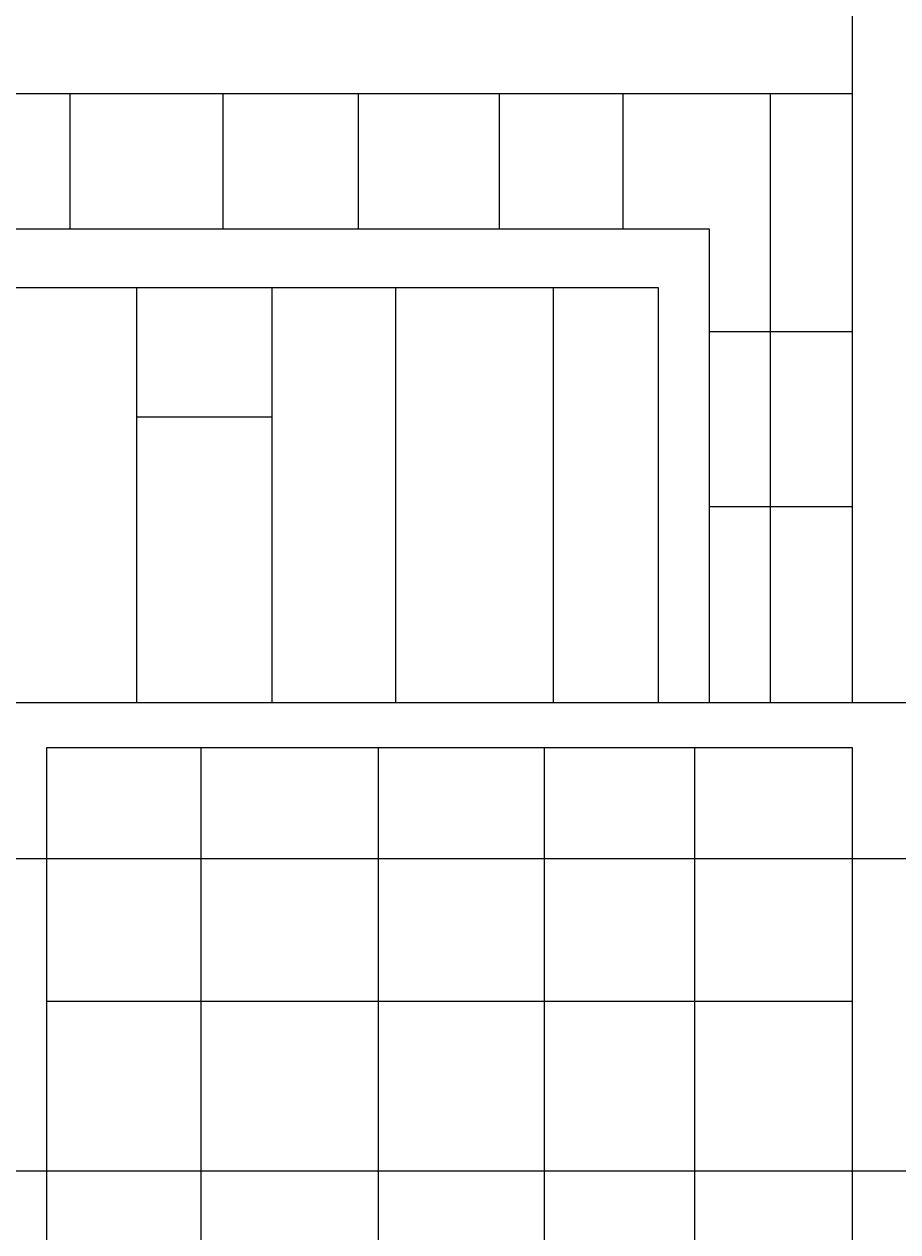
# Model space of a CAD drawing. Units: inches. Extents: x -117 to 121, y -77 to 40.
# Tile 14 of 45: x -45 to -23, y -23 to 7. Entities that reach past the tile are written whole.
import ezdxf

# ---------------------------------------------------------------- set-up
doc = ezdxf.new("R2010")
doc.units = ezdxf.units.IN
doc.header["$MEASUREMENT"] = 0
doc.layers.add('A-ANNO-DIMS', color=2, linetype='Continuous', lineweight=18)
doc.layers.add('A-ELEV', color=7, linetype='Continuous', lineweight=25)
doc.styles.get("Standard").update_dxf_attribs({"font": 'arial.ttf'})
doc.dimstyles.get("Standard").update_dxf_attribs({"dimtxt": 0.18, "dimasz": 0.18, "dimexe": 0.18, "dimexo": 0.0625, "dimgap": 0.09, "dimtad": 0, "dimtih": 1, "dimtoh": 1, "dimdec": 4, "dimzin": 0, "dimdsep": 46, "dimtxsty": 'Standard', "dimcen": 0.09, "dimadec": 0, "dimazin": 0, "dimtfac": 1, "dimtdec": 4, "dimtofl": 0, "dimtmove": 0, "dimatfit": 3, "dimfxl": 1, "dimtolj": 1, "dimtzin": 0, "dimarcsym": 0})

# ---------------------------------------------------------------- blocks, each defined once
blk = doc.blocks.new('*D13')
at = {"layer": 'A-ANNO-DIMS', "color": 0, "lineweight": -2, "transparency": 16777216}
for p, q in [((-2.663, 27.063), (-117.024, 27.063)), ((-116.844, 26.883), (-116.844, -16.974)), ((-116.844, -61.196), (-116.844, -17.338)), ((-106.096, -61.376), (-117.024, -61.376))]:
    blk.add_line(p, q, dxfattribs=at)
at = {"layer": 'A-ANNO-DIMS', "color": 0, "transparency": 16777216}
for points in [[(-116.874, 26.883), (-116.814, 26.883), (-116.844, 27.063)], [(-116.874, -61.196), (-116.814, -61.196), (-116.844, -61.376)]]:
    blk.add_solid(points, dxfattribs=at)
at = {"layer": 'Defpoints', "color": 0, "transparency": 16777216}
for p in [(-2.6, 27.063), (-116.844, -61.376), (-106.034, -61.376)]:
    blk.add_point(p, dxfattribs=at)
at = {"layer": 'A-ANNO-DIMS', "color": 0, "transparency": 16777216, "insert": (-116.844, -17.156), "char_height": 0.18, "attachment_point": 5}
blk.add_mtext('\\A1;88.44', dxfattribs=at)
blk = doc.blocks.new('*D50')
at = {"layer": 'A-ANNO-DIMS', "color": 0, "lineweight": -2, "transparency": 16777216}
for p, q in [((-47.458, -13.74), (120.84, -13.74)), ((120.66, -13.92), (120.66, -17.512)), ((120.66, -21.468), (120.66, -17.876)), ((-47.458, -21.648), (120.84, -21.648))]:
    blk.add_line(p, q, dxfattribs=at)
at = {"layer": 'A-ANNO-DIMS', "color": 0, "transparency": 16777216}
for points in [[(120.63, -13.92), (120.69, -13.92), (120.66, -13.74)], [(120.63, -21.468), (120.69, -21.468), (120.66, -21.648)]]:
    blk.add_solid(points, dxfattribs=at)
at = {"layer": 'Defpoints', "color": 0, "transparency": 16777216}
for p in [(-47.521, -13.74), (120.66, -13.74), (-47.521, -21.648)]:
    blk.add_point(p, dxfattribs=at)
at = {"layer": 'A-ANNO-DIMS', "color": 0, "transparency": 16777216, "insert": (120.66, -17.694), "char_height": 0.18, "attachment_point": 5}
blk.add_mtext('\\A1;7.908', dxfattribs=at)

msp = doc.modelspace()

# ---------------------------------------------------------------- linework, layer by layer
at = {"layer": 'A-ELEV'}
for p, q in [((-23.8637, 14.0735), (-23.8637, 2.5407)), ((-23.8637, 5.6231), (-74.3507, 5.6231)), ((-43.6654, 2.2073), (-43.6654, 5.6231)), ((-39.7925, 2.2073), (-39.7925, 5.6231)), ((-36.3665, 2.2073), (-36.3665, 5.6231)), ((-32.7915, 2.2073), (-32.7915, 5.6231)), ((-29.6634, 2.2073), (-29.6634, 5.6231)), ((-25.9369, -9.7904), (-25.9369, 5.6231)), ((-23.8637, 2.5407), (-23.8637, -9.7904)), ((-64.513, 2.2073), (-27.4892, 2.2073)), ((-27.4892, 2.2073), (-27.4892, -9.7904)), ((-28.7689, 0.7128), (-63.0775, 0.7128)), ((-41.9822, 0.7128), (-41.9822, -9.7904)), ((-38.5613, 0.7128), (-38.5613, -9.7904)), ((-35.4255, 0.7128), (-35.4255, -9.7904)), ((-31.4345, 0.7128), (-31.4345, -9.7904)), ((-28.7689, -9.7904), (-28.7689, 0.7128)), ((-27.4892, -0.3942), (-23.8637, -0.3942)), ((-41.9822, -2.551), (-38.5613, -2.551)), ((-27.4892, -4.8248), (-23.8637, -4.8248)), ((-45.4848, -9.7904), (-23.8637, -9.7904)), ((-23.8637, -9.7904), (-22.4056, -9.7904)), ((-44.2539, -23.5007), (-44.2539, -10.9315)), ((-44.2539, -10.9315), (-23.8637, -10.9315)), ((-40.3483, -23.5007), (-40.3483, -10.9315)), ((-35.8568, -23.5007), (-35.8568, -10.9315)), ((-31.6582, -23.5007), (-31.6582, -10.9315)), ((-27.8502, -23.5007), (-27.8502, -10.9315)), ((-23.8637, -10.9315), (-23.8637, -14.3771)), ((-23.8637, -14.3771), (-23.8637, -23.5007)), ((-23.8637, -17.3566), (-44.2539, -17.3566))]:
    msp.add_line(p, q, dxfattribs=at)

# ---------------------------------------------------------------- dimensions: what is measured, and where the dimension line sits
at = {"layer": 'A-ANNO-DIMS'}
for base, p1, p2, override, picture, middle in [((-116.8438, -61.3756), (-2.6001, 27.0634), (-106.0338, -61.3756), {"dimdec": 2, "dimlfac": 1, "dimrnd": 0, "dimzin": 0, "dimdsep": 46, "dimlunit": 2}, '*D13', (-116.8438, -17.1561)), ((120.6602, -13.74), (-47.5206, -21.6476), (-47.5206, -13.74), {"dimdec": 3, "dimlfac": 1, "dimrnd": 0, "dimzin": 0, "dimdsep": 46, "dimlunit": 2}, '*D50', (120.6602, -17.6938))]:
    dim = msp.add_linear_dim(base=base, p1=p1, p2=p2, angle=90, dimstyle='Standard', override=override, dxfattribs=at)
    dim.commit()
    dim.dimension.update_dxf_attribs({"geometry": picture, "text_midpoint": middle})

doc.saveas('drawing.dxf')
